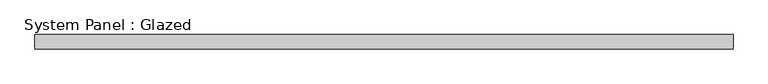
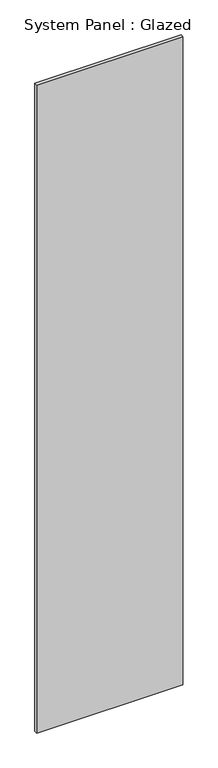
"""IFC4 building model written with IfcOpenShell, lengths in millimetres: plate geometry, System Panel : Glazed."""

from ifc_helpers import new_model, si_unit, origin, origin_with_axes, place, context, project, spatial, polyline, outline, extrude, source, transform, mapped, element, save


def system_panel_glazed_3f11bb86(model_context):
    return source(origin(), model_context, "Body", "SweptSolid", [
        extrude(outline(polyline([(628.65, 19.05), (-628.65, 19.05), (-628.65, 44.45), (628.65, 44.45), (628.65, 19.05)])), origin_with_axes(), (0.0, 0.0, 1.0), 5884.7116741),
    ])


if __name__ == "__main__":
    model = new_model("IFC4")
    model_context = context("Model", 3, world=origin())
    ifc_project = project(units=[si_unit("LENGTHUNIT", "METRE", prefix="MILLI")], contexts=[model_context])
    site = spatial("IfcSite", under=ifc_project)
    building = spatial("IfcBuilding", under=site)
    placement = place(None, origin())
    system_panel_glazed_shape = system_panel_glazed_3f11bb86(model_context)
    element("IfcPlate", 1, ObjectType="System Panel : Glazed", at=placement, inside=building, context=model_context, shape_type="MappedRepresentation", body=[
        mapped(system_panel_glazed_shape, transform((0.0, 0.0, 0.0), x_axis=(1.0, 0.0, 0.0), y_axis=(0.0, 1.0, 0.0), z_axis=(0.0, 0.0, 1.0))),
    ])
    save(model, "model.ifc")

# Revit data of these elements
# Type "System Panel : Glazed"
#   Construction Type Id = "GSP4R"
#   Analytic Construction = "1/8 in Pilkington single glazing"
#   Visual Light Transmittance = 0.9
#   Solar Heat Gain Coefficient = 0.86
#   Heat Transfer Coefficient (U) = 1.18115 BTU/(h·ft²·°F)
# Element 1 (IfcPlate, "System Panel : Glazed")
#   Materials on its faces: "Glass"
# Materials
#   "Glass": class "Glass", colour RGB 0 128 192, transparency 0.75, Description = "Soda Lime Glass", Cost = 0
